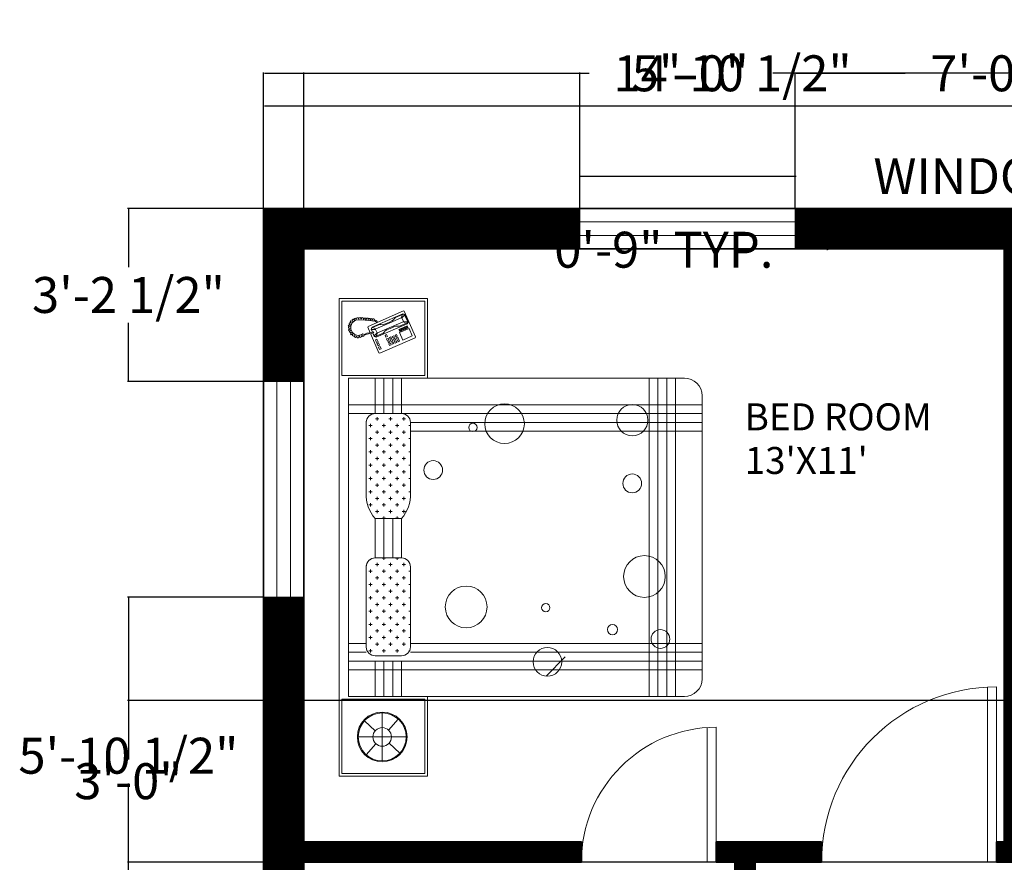
# Model space of a CAD drawing. Units: inches. Extents: x 108 to 771, y 58 to 590.
# Tile 5 of 8: x 108 to 327, y 402 to 590. Entities that reach past the tile are written whole.
import ezdxf

# ---------------------------------------------------------------- set-up
doc = ezdxf.new("R2010")
doc.units = ezdxf.units.IN
doc.header["$MEASUREMENT"] = 0
for name, color, linetype, lineweight in [('A-ANNO-DIMS', 2, 'Continuous', 13), ('A-AREA-IDEN', 7, 'Continuous', 18), ('A-DOOR', 3, 'Continuous', 18), ('A-GLAZ', 4, 'Continuous', 18), ('A-WALL', 7, 'Continuous', 35), ('A-WALL-PATT', 252, 'Continuous', 9), ('Furniture', 7, 'Continuous', 15)]:
    doc.layers.add(name, color=color, linetype=linetype, lineweight=lineweight)
doc.styles.get("Standard").update_dxf_attribs({"font": 'italic8.shx'})
doc.dimstyles.get("Standard").update_dxf_attribs({"dimtxt": 8, "dimasz": 0.18, "dimexe": 0.18, "dimexo": 0.0625, "dimgap": 0.09, "dimtad": 0, "dimtih": 1, "dimtoh": 1, "dimzin": 0, "dimdsep": 46, "dimlunit": 3, "dimtxsty": 'Standard', "dimcen": 0.09, "dimclrt": 6, "dimadec": 0, "dimazin": 0, "dimtfac": 1, "dimtofl": 0, "dimtmove": 0, "dimatfit": 3, "dimfxl": 1, "dimtolj": 1, "dimtzin": 0, "dimarcsym": 0})

# ---------------------------------------------------------------- blocks, each defined once
blk = doc.blocks.new('*D5')
at = {"layer": 'A-ANNO-DIMS', "color": 0, "lineweight": -2, "transparency": 16777216}
for p, q in [((162.35, 548.12), (162.35, 571.05)), ((162.53, 570.87), (386.42, 570.87)), ((677.17, 570.87), (453.27, 570.87)), ((677.35, 548.12), (677.35, 571.05))]:
    blk.add_line(p, q, dxfattribs=at)
at = {"layer": 'A-ANNO-DIMS', "color": 0, "transparency": 16777216}
for points in [[(162.53, 570.9), (162.53, 570.84), (162.35, 570.87)], [(677.17, 570.9), (677.17, 570.84), (677.35, 570.87)]]:
    blk.add_solid(points, dxfattribs=at)
at = {"layer": 'Defpoints', "color": 0, "transparency": 16777216}
for p in [(677.35, 570.87), (162.35, 548.05), (677.35, 548.05)]:
    blk.add_point(p, dxfattribs=at)
at = {"layer": 'A-ANNO-DIMS', "color": 0, "transparency": 16777216, "insert": (419.85, 570.87), "char_height": 8, "attachment_point": 5}
blk.add_mtext('\\A1;42\'-11.00"', dxfattribs=at)
blk = doc.blocks.new('DOOR-SINGLE-39')
for p, q in [((0, 39), (0, 0)), ((2, 38.95), (2, 0)), ((0, 0), (39, 0))]:
    blk.add_line(p, q)
blk.add_arc((0, 0), 39, 0, 90)
blk = doc.blocks.new('DOOR-SINGLE-30')
for p, q in [((28, 29.93), (28, 0)), ((30, 30), (30, 0)), ((30, 0), (0, 0))]:
    blk.add_line(p, q)
blk.add_arc((30, 0), 30, 90, 180)
blk = doc.blocks.new('WINDOW-48')
for p, q in [((0, 48), (0, 0)), ((9, 48), (0, 48)), ((3, 48), (3, 0)), ((6, 48), (6, 0)), ((9, 0), (9, 48)), ((0, 0), (9, 0))]:
    blk.add_line(p, q)
blk = doc.blocks.new('BED-WITH-NIGHTSTANDS')
h = blk.add_hatch()
h.set_pattern_fill('CROSS', color=256, scale=5.9055, angle=450, style=0)
h.set_pattern_definition([(90, (-724.7189, -618.2251), (1.476375, 1.476375), [0.7381875, -2.2145625]), (360, (-725.088, -617.856), (1.476375, -1.476375), [0.7381875, -2.2145625])])
h.paths.add_polyline_path([(13.93, 48.57), (8.02, 48.57, 0.414214), (6.06, 46.6), (6.06, 28.74, 0.414214), (8.02, 26.77), (13.93, 26.77, 0.414214), (15.9, 28.74), (15.9, 46.6, 0.414214)])
h.paths.add_polyline_path([(6.06, 62.99, 0.19223), (8.02, 57.33), (13.93, 57.33, 0.19223), (15.9, 62.99), (15.9, 78.74, 0.414214), (13.93, 80.71), (8.02, 80.71, 0.414214), (6.06, 78.74)])
for p, q in [((0, 0), (0, 106.3)), ((19.69, 106.3), (0, 106.3)), ((19.09, 105.71), (0.59, 105.71)), ((0.59, 105.71), (0.59, 89.17)), ((19.09, 105.71), (19.09, 89.17)), ((19.69, 106.3), (19.69, 88.58)), ((14.35, 103.55), (6.45, 100.09)), ((14.52, 103.48), (14.35, 103.55)), ((17.02, 97.76), (14.52, 103.48)), ((2.23, 100.67), (2.3, 100.88)), ((2.3, 100.88), (2.69, 100.86)), ((2.44, 101.15), (2.63, 101.34)), ((2.69, 100.86), (2.44, 101.15)), ((2.89, 100.92), (2.62, 100.19)), ((2.63, 101.34), (3.06, 101.2)), ((2.89, 101.55), (3.11, 101.7)), ((3.06, 101.2), (2.89, 101.55)), ((3.69, 101.46), (2.89, 100.92)), ((3.11, 101.7), (3.41, 101.48)), ((3.36, 101.88), (3.67, 101.95)), ((3.41, 101.48), (3.36, 101.88)), ((3.67, 101.95), (3.81, 101.64)), ((4.95, 101.56), (3.69, 101.46)), ((3.81, 101.64), (3.94, 101.98)), ((3.94, 101.98), (4.24, 102.02)), ((4.24, 102.02), (4.39, 101.64)), ((4.37, 102.03), (4.76, 102.08)), ((4.39, 101.64), (4.37, 102.03)), ((4.76, 102.08), (4.88, 101.72)), ((4.88, 101.72), (5.13, 102.07)), ((5.79, 101.48), (4.95, 101.56)), ((5.13, 102.07), (5.37, 102.03)), ((5.37, 102.03), (5.42, 101.66)), ((5.42, 101.66), (5.65, 101.97)), ((5.65, 101.97), (5.95, 101.95)), ((5.86, 101.55), (5.79, 101.48)), ((5.92, 101.48), (5.86, 101.55)), ((6.5, 101.45), (5.92, 101.48)), ((5.95, 101.95), (5.98, 101.59)), ((5.98, 101.59), (6.16, 101.92)), ((6.16, 101.92), (6.47, 101.91)), ((6.47, 101.91), (6.46, 101.54)), ((6.46, 101.54), (6.62, 101.9)), ((7.29, 101.35), (6.5, 101.45)), ((6.62, 101.9), (6.85, 101.89)), ((6.85, 101.89), (6.89, 101.51)), ((6.89, 101.51), (7.15, 101.84)), ((7.15, 101.84), (7.36, 101.82)), ((7.73, 101.29), (7.29, 101.35)), ((14.21, 102.94), (7.34, 99.94)), ((7.36, 101.82), (7.4, 101.48)), ((7.4, 101.48), (7.62, 101.8)), ((7.62, 101.8), (7.77, 101.81)), ((7.79, 101.48), (7.73, 101.29)), ((7.77, 101.81), (7.86, 101.7)), ((7.84, 101.37), (7.79, 101.48)), ((7.94, 101.33), (7.84, 101.37)), ((7.86, 101.7), (7.96, 101.49)), ((8.11, 101.22), (7.94, 101.33)), ((7.96, 101.49), (8.25, 101.43)), ((8.26, 101.14), (8.11, 101.22)), ((11.28, 100.91), (8.18, 99.56)), ((8.25, 101.43), (8.4, 101.32)), ((8.4, 100.95), (8.26, 101.14)), ((8.4, 101.32), (8.57, 101.02)), ((10.11, 100.6), (11.2, 101.08)), ((11.77, 101.33), (11.2, 101.08)), ((11.28, 100.91), (13.85, 102.03)), ((11.68, 99.99), (14.25, 101.12)), ((12.15, 101.56), (11.77, 101.33)), ((12.36, 101.86), (12.15, 101.56)), ((12.6, 102.1), (12.36, 101.86)), ((14.14, 102.78), (12.6, 102.1)), ((14.14, 102.78), (13.85, 102.03)), ((13.85, 102.03), (13.99, 102.03)), ((13.99, 102.03), (14.61, 102.64)), ((13.99, 102.03), (14.34, 101.23)), ((14.4, 102.82), (14.14, 102.78)), ((14.62, 102.78), (14.21, 102.94)), ((14.25, 101.12), (14.34, 101.23)), ((15, 100.83), (14.25, 101.12)), ((14.34, 101.23), (15.21, 101.26)), ((14.61, 102.64), (14.4, 102.82)), ((15.21, 101.26), (14.61, 102.64)), ((15.37, 101.06), (14.62, 102.78)), ((15.2, 100.99), (15, 100.83)), ((15.18, 100.71), (15.37, 101.06)), ((15.21, 101.26), (15.2, 100.99)), ((2.06, 100.15), (2.14, 100.41)), ((2.46, 100.04), (2.06, 100.15)), ((2.09, 99.7), (2.1, 99.92)), ((2.44, 99.53), (2.09, 99.7)), ((2.1, 99.92), (2.46, 100.04)), ((2.13, 99.38), (2.44, 99.53)), ((2.17, 99.14), (2.13, 99.38)), ((2.14, 100.41), (2.51, 100.41)), ((2.59, 99.17), (2.17, 99.14)), ((2.51, 100.41), (2.23, 100.67)), ((2.29, 98.95), (2.59, 99.17)), ((2.4, 98.76), (2.29, 98.95)), ((2.78, 98.76), (2.4, 98.76)), ((2.53, 98.47), (2.78, 98.76)), ((2.62, 100.19), (2.62, 99.39)), ((2.62, 99.39), (2.98, 98.72)), ((2.98, 98.72), (3.58, 98.25)), ((6.45, 100.09), (6.38, 99.93)), ((6.38, 99.93), (6.92, 98.7)), ((6.77, 98.66), (7.17, 98.75)), ((7.34, 99.94), (7.12, 99.5)), ((7.12, 99.5), (7.41, 98.83)), ((7.17, 98.75), (7.65, 98.91)), ((7.72, 98.74), (7.22, 98.53)), ((7.23, 99.41), (7.24, 99.69)), ((8.09, 99.45), (7.23, 99.41)), ((7.47, 98.85), (7.23, 99.41)), ((7.24, 99.69), (7.44, 99.85)), ((7.44, 99.85), (8.99, 100.52)), ((7.44, 99.85), (8.18, 99.56)), ((7.65, 98.91), (7.72, 98.74)), ((8.18, 99.56), (8.09, 99.45)), ((8.09, 99.45), (8.45, 98.65)), ((8.26, 97.68), (15.18, 100.71)), ((11.68, 99.99), (8.58, 98.64)), ((8.99, 100.52), (9.33, 100.53)), ((9.33, 100.53), (9.69, 100.49)), ((9.69, 100.49), (10.11, 100.6)), ((9.84, 98.58), (10.08, 98.82)), ((10.08, 98.82), (10.29, 99.11)), ((10.29, 99.11), (10.66, 99.34)), ((10.66, 99.34), (11.75, 99.82)), ((12.33, 100.07), (11.75, 99.82)), ((12.75, 100.19), (12.33, 100.07)), ((13.11, 100.14), (12.75, 100.19)), ((13.45, 100.15), (13.11, 100.14)), ((13.3, 99.4), (13.47, 99.48)), ((13.5, 98.95), (13.3, 99.4)), ((15, 100.83), (13.45, 100.15)), ((15.58, 99.65), (13.46, 98.72)), ((13.46, 98.72), (14.18, 97.06)), ((13.47, 99.48), (13.67, 99.02)), ((13.67, 99.02), (13.5, 98.95)), ((13.64, 99.55), (13.81, 99.63)), ((13.84, 99.1), (13.64, 99.55)), ((13.81, 99.63), (14.01, 99.17)), ((14.01, 99.17), (13.84, 99.1)), ((13.99, 99.7), (14.16, 99.78)), ((14.19, 99.25), (13.99, 99.7)), ((14.16, 99.78), (14.36, 99.32)), ((14.36, 99.32), (14.19, 99.25)), ((14.33, 99.85), (14.5, 99.93)), ((14.53, 99.4), (14.33, 99.85)), ((14.5, 99.93), (14.7, 99.47)), ((14.7, 99.47), (14.53, 99.4)), ((14.67, 100), (14.84, 100.08)), ((14.87, 99.55), (14.67, 100)), ((14.84, 100.08), (15.04, 99.62)), ((15.04, 99.62), (14.87, 99.55)), ((15.02, 100.16), (15.19, 100.23)), ((15.22, 99.7), (15.02, 100.16)), ((15.19, 100.23), (15.39, 99.77)), ((15.39, 99.77), (15.22, 99.7)), ((16.3, 97.99), (15.58, 99.65)), ((2.71, 98.26), (2.53, 98.47)), ((3.07, 98.46), (2.71, 98.26)), ((2.96, 98.08), (3.07, 98.46)), ((3.2, 97.92), (2.96, 98.08)), ((3.49, 98.1), (3.2, 97.92)), ((3.41, 97.75), (3.49, 98.1)), ((3.69, 97.67), (3.41, 97.75)), ((3.58, 98.25), (4.33, 98.05)), ((3.95, 97.97), (3.69, 97.67)), ((4.03, 97.59), (3.95, 97.97)), ((4.36, 97.56), (4.03, 97.59)), ((4.33, 98.05), (5.08, 98.31)), ((4.48, 97.99), (4.36, 97.56)), ((4.67, 97.64), (4.48, 97.99)), ((5, 97.75), (4.67, 97.64)), ((5.05, 98.16), (5, 97.75)), ((5.26, 97.85), (5.05, 98.16)), ((5.08, 98.31), (5.33, 98.48)), ((5.53, 98), (5.26, 97.85)), ((5.33, 98.48), (5.57, 98.34)), ((5.6, 98.18), (5.53, 98)), ((5.57, 98.34), (5.87, 98.48)), ((5.68, 98.18), (5.6, 98.18)), ((5.98, 98.32), (5.68, 98.18)), ((5.87, 98.48), (6.16, 98.57)), ((6.58, 98.42), (5.98, 98.32)), ((6.16, 98.57), (6.77, 98.66)), ((7.22, 98.53), (6.58, 98.42)), ((7.01, 98.5), (8.89, 94.2)), ((7.49, 98.64), (7.84, 97.84)), ((7.83, 98.04), (7.55, 98.67)), ((8.45, 98.65), (7.83, 98.04)), ((7.83, 98.04), (8.04, 97.86)), ((7.84, 97.84), (8.26, 97.68)), ((8.04, 97.86), (8.29, 97.9)), ((8.09, 97.13), (8.43, 97.28)), ((8.34, 96.55), (8.09, 97.13)), ((8.29, 97.9), (8.58, 98.64)), ((8.29, 97.9), (9.84, 98.58)), ((8.68, 96.7), (8.34, 96.55)), ((8.43, 97.28), (8.68, 96.7)), ((8.58, 98.64), (8.45, 98.65)), ((9.05, 94.14), (16.96, 97.59)), ((10.58, 98.29), (10.24, 98.14)), ((10.24, 98.14), (10.44, 97.68)), ((10.44, 97.68), (10.78, 97.83)), ((10.78, 97.83), (10.58, 98.29)), ((10.93, 97.48), (10.59, 97.33)), ((10.59, 97.33), (10.74, 96.99)), ((10.74, 96.99), (11.08, 97.14)), ((11.18, 96.91), (10.84, 96.76)), ((10.84, 96.76), (10.99, 96.42)), ((11.08, 97.14), (10.93, 97.48)), ((10.99, 96.42), (11.33, 96.57)), ((11.33, 96.57), (11.18, 96.91)), ((11.56, 97.76), (11.22, 97.61)), ((11.22, 97.61), (11.37, 97.27)), ((11.37, 97.27), (11.71, 97.42)), ((11.81, 97.19), (11.47, 97.04)), ((11.47, 97.04), (11.62, 96.69)), ((11.71, 97.42), (11.56, 97.76)), ((11.62, 96.69), (11.96, 96.84)), ((12.06, 96.61), (11.72, 96.46)), ((11.96, 96.84), (11.81, 97.19)), ((12.19, 98.03), (11.85, 97.88)), ((11.85, 97.88), (12, 97.54)), ((12, 97.54), (12.34, 97.69)), ((12.21, 96.27), (12.06, 96.61)), ((12.44, 97.46), (12.1, 97.31)), ((12.1, 97.31), (12.25, 96.97)), ((12.34, 97.69), (12.19, 98.03)), ((12.25, 96.97), (12.59, 97.12)), ((12.69, 96.89), (12.35, 96.74)), ((12.35, 96.74), (12.5, 96.39)), ((12.59, 97.12), (12.44, 97.46)), ((12.82, 98.31), (12.48, 98.16)), ((12.48, 98.16), (12.63, 97.82)), ((12.5, 96.39), (12.84, 96.55)), ((12.63, 97.82), (12.97, 97.97)), ((12.84, 96.55), (12.69, 96.89)), ((13.07, 97.74), (12.73, 97.59)), ((12.73, 97.59), (12.88, 97.24)), ((12.97, 97.97), (12.82, 98.31)), ((12.88, 97.24), (13.22, 97.39)), ((13.32, 97.16), (12.98, 97.01)), ((12.98, 97.01), (13.13, 96.67)), ((13.22, 97.39), (13.07, 97.74)), ((13.13, 96.67), (13.47, 96.82)), ((13.47, 96.82), (13.32, 97.16)), ((14.18, 97.06), (16.3, 97.99)), ((16.96, 97.59), (17.02, 97.76)), ((8.44, 96.33), (8.78, 96.48)), ((8.69, 95.75), (8.44, 96.33)), ((9.03, 95.9), (8.69, 95.75)), ((8.78, 96.48), (9.03, 95.9)), ((8.79, 95.52), (9.13, 95.67)), ((9.04, 94.95), (8.79, 95.52)), ((9.38, 95.1), (9.04, 94.95)), ((9.13, 95.67), (9.38, 95.1)), ((11.43, 96.34), (11.09, 96.19)), ((11.09, 96.19), (11.24, 95.84)), ((11.24, 95.84), (11.58, 95.99)), ((11.58, 95.99), (11.43, 96.34)), ((11.72, 96.46), (11.87, 96.12)), ((11.87, 96.12), (12.21, 96.27)), ((8.89, 94.2), (9.05, 94.14)), ((19.09, 89.17), (0.59, 89.17)), ((0.59, 89.17), (19.09, 89.17)), ((2.12, 17.72), (2.12, 88.58)), ((2.12, 88.58), (76.92, 88.58)), ((80.86, 84.65), (80.86, 21.65)), ((55.34, 82.68), (55.28, 82.62)), ((6.07, 78.98), (6.07, 62.76)), ((6.07, 46.84), (6.07, 28.51)), ((6.07, 44.57), (6.06, 44.56)), ((50.36, 26.51), (46.1, 22.26)), ((76.92, 17.72), (2.12, 17.72)), ((19.69, 0), (19.69, 17.72)), ((19.09, 17.13), (0.59, 17.13)), ((0.59, 0.59), (0.59, 17.13)), ((19.09, 0.59), (19.09, 17.13)), ((9.61, 8.71), (9.61, 14.05)), ((8.07, 10.1), (5.65, 12.3)), ((11, 10.24), (13.2, 12.67)), ((9.61, 8.71), (4.26, 8.71)), ((8.22, 7.18), (6.02, 4.75)), ((9.61, 8.71), (14.95, 8.71)), ((9.61, 8.71), (9.61, 3.36)), ((11.14, 7.32), (13.56, 5.12)), ((19.69, 0), (0, 0)), ((19.09, 0.59), (0.59, 0.59))]:
    blk.add_line(p, q)
for points in [[(8.02, 88.58), (8.02, 80.71)], [(9.99, 80.71), (9.99, 88.58), (8.02, 88.58)], [(13.93, 80.71), (13.93, 88.58), (11.96, 88.58)], [(11.96, 88.58), (11.96, 80.71)], [(2.12, 80.71), (80.86, 80.71), (80.86, 82.68), (2.12, 82.68)], [(15.9, 76.77), (80.86, 76.77), (80.86, 78.74), (15.9, 78.74)], [(8.02, 57.33), (8.02, 48.57)], [(9.99, 48.57), (9.99, 57.33)], [(11.96, 57.33), (11.96, 48.57)], [(13.93, 48.57), (13.93, 57.33)], [(2.12, 29.53), (6.06, 29.53)], [(15.9, 29.53), (80.86, 29.53), (80.86, 27.56), (15.9, 27.56)], [(6.06, 27.56), (2.12, 27.56)], [(2.12, 25.59), (80.86, 25.59), (80.86, 23.62), (2.12, 23.62)], [(8.02, 25.59), (8.02, 17.72), (9.99, 17.72), (9.99, 25.59)], [(11.96, 25.59), (11.96, 17.72), (13.93, 17.72), (13.93, 25.59)]]:
    blk.add_lwpolyline(points)
for points in [[(69.05, 88.58), (69.05, 17.72), (71.02, 17.72), (71.02, 88.58)], [(72.98, 88.58), (72.98, 17.72), (74.95, 17.72), (74.95, 88.58)]]:
    blk.add_lwpolyline(points, close=True)
for points in [[(15.9, 62.99), (15.9, 78.74, 0.414214), (13.93, 80.71), (8.02, 80.71, 0.414214), (6.06, 78.74), (6.06, 62.99, 0.19223), (8.02, 57.33), (13.93, 57.33, 0.19223)], [(15.9, 28.74), (15.9, 46.6, 0.414214), (13.93, 48.57), (8.02, 48.57, 0.414214), (6.06, 46.6), (6.06, 28.74, 0.414214), (8.02, 26.77), (13.93, 26.77, 0.414214)]]:
    blk.add_lwpolyline(points, format="xyb", close=True)
for centre, radius in [((36.86, 78.44), 4.41), ((65.32, 79.25), 3.48), ((29.81, 77.62), 0.925), ((20.97, 68.13), 2.09), ((65.3, 65.16), 2.09), ((68.02, 44.43), 4.65), ((28.31, 37.66), 4.65), ((46.05, 37.48), 0.925), ((60.91, 32.6), 1.14), ((71.58, 30.51), 2.09), ((46.4, 25.43), 3.19), ((9.61, 8.71), 5.54), ((9.61, 8.71), 5.34), ((9.61, 8.71), 2.07)]:
    blk.add_circle(centre, radius)
for centre, start, end in [((76.92, 84.65), 0, 90), ((76.92, 21.65), 270, 0)]:
    blk.add_arc(centre, 3.94, start, end)
blk = doc.blocks.new('*D20')
at = {"layer": 'A-ANNO-DIMS', "color": 0, "lineweight": -2, "transparency": 16777216}
for p, q in [((232.77, 548.12), (232.77, 555.43)), ((232.95, 555.25), (280.59, 555.25)), ((280.77, 548.12), (280.77, 555.43)), ((280.77, 555.25), (280.95, 555.25))]:
    blk.add_line(p, q, dxfattribs=at)
at = {"layer": 'A-ANNO-DIMS', "color": 0, "transparency": 16777216}
for points in [[(232.95, 555.28), (232.95, 555.22), (232.77, 555.25)], [(280.59, 555.28), (280.59, 555.22), (280.77, 555.25)]]:
    blk.add_solid(points, dxfattribs=at)
at = {"layer": 'Defpoints', "color": 0, "transparency": 16777216}
for p in [(280.77, 555.25), (232.77, 548.05), (280.77, 548.05)]:
    blk.add_point(p, dxfattribs=at)
at = {"layer": 'A-ANNO-DIMS', "color": 6, "transparency": 16777216, "insert": (346.76, 555.25), "char_height": 8, "attachment_point": 5}
blk.add_mtext('\\A1;WINDOW 4\'-0" TYP.', dxfattribs=at)
blk = doc.blocks.new('*D21')
at = {"layer": 'A-ANNO-DIMS', "color": 0, "lineweight": -2, "transparency": 16777216}
for p, q in [((280.83, 548.05), (288.15, 548.05)), ((287.97, 547.87), (287.97, 539.23)), ((280.83, 539.05), (288.15, 539.05)), ((287.97, 538.87), (287.79, 538.87)), ((287.97, 539.05), (287.97, 538.87))]:
    blk.add_line(p, q, dxfattribs=at)
at = {"layer": 'A-ANNO-DIMS', "color": 0, "transparency": 16777216}
for points in [[(287.94, 547.87), (288, 547.87), (287.97, 548.05)], [(287.94, 539.23), (288, 539.23), (287.97, 539.05)]]:
    blk.add_solid(points, dxfattribs=at)
at = {"layer": 'Defpoints', "color": 0, "transparency": 16777216}
for p in [(280.77, 548.05), (280.77, 539.05), (287.97, 539.05)]:
    blk.add_point(p, dxfattribs=at)
at = {"layer": 'A-ANNO-DIMS', "color": 6, "transparency": 16777216, "insert": (251.51, 538.87), "char_height": 8, "attachment_point": 5}
blk.add_mtext('\\A1;0\'-9" TYP.', dxfattribs=at)
blk = doc.blocks.new('*D53')
at = {"layer": 'A-ANNO-DIMS', "color": 0, "lineweight": -2, "transparency": 16777216}
for p, q in [((162.35, 548.12), (162.35, 578.33)), ((162.53, 578.15), (232.59, 578.15)), ((232.77, 548.12), (232.77, 578.33)), ((232.77, 578.15), (232.95, 578.15))]:
    blk.add_line(p, q, dxfattribs=at)
at = {"layer": 'A-ANNO-DIMS', "color": 0, "transparency": 16777216}
for points in [[(162.53, 578.18), (162.53, 578.12), (162.35, 578.15)], [(232.59, 578.18), (232.59, 578.12), (232.77, 578.15)]]:
    blk.add_solid(points, dxfattribs=at)
at = {"layer": 'Defpoints', "color": 0, "transparency": 16777216}
for p in [(232.77, 578.15), (162.35, 548.05), (232.77, 548.05)]:
    blk.add_point(p, dxfattribs=at)
at = {"layer": 'A-ANNO-DIMS', "color": 6, "transparency": 16777216, "insert": (268.85, 578.15), "char_height": 8, "attachment_point": 5}
blk.add_mtext('\\A1;5\'-10 1/2"', dxfattribs=at)
blk = doc.blocks.new('*D54')
at = {"layer": 'A-ANNO-DIMS', "color": 0, "lineweight": -2, "transparency": 16777216}
for p, q in [((280.77, 548.12), (280.77, 578.33)), ((280.95, 578.15), (305.28, 578.15)), ((364.84, 578.15), (340.51, 578.15)), ((365.02, 548.12), (365.02, 578.33))]:
    blk.add_line(p, q, dxfattribs=at)
at = {"layer": 'A-ANNO-DIMS', "color": 0, "transparency": 16777216}
for points in [[(280.95, 578.18), (280.95, 578.12), (280.77, 578.15)], [(364.84, 578.18), (364.84, 578.12), (365.02, 578.15)]]:
    blk.add_solid(points, dxfattribs=at)
at = {"layer": 'Defpoints', "color": 0, "transparency": 16777216}
for p in [(365.02, 578.15), (280.77, 548.05), (365.02, 548.05)]:
    blk.add_point(p, dxfattribs=at)
at = {"layer": 'A-ANNO-DIMS', "color": 6, "transparency": 16777216, "insert": (322.9, 578.15), "char_height": 8, "attachment_point": 5}
blk.add_mtext('\\A1;7\'-0"', dxfattribs=at)
blk = doc.blocks.new('*D57')
at = {"layer": 'A-ANNO-DIMS', "color": 0, "lineweight": -2, "transparency": 16777216}
for p, q in [((162.28, 548.05), (132.07, 548.05)), ((132.25, 547.87), (132.25, 534.99)), ((132.25, 509.73), (132.25, 522.62)), ((171.28, 509.55), (132.07, 509.55))]:
    blk.add_line(p, q, dxfattribs=at)
at = {"layer": 'A-ANNO-DIMS', "color": 0, "transparency": 16777216}
for points in [[(132.22, 547.87), (132.28, 547.87), (132.25, 548.05)], [(132.22, 509.73), (132.28, 509.73), (132.25, 509.55)]]:
    blk.add_solid(points, dxfattribs=at)
at = {"layer": 'Defpoints', "color": 0, "transparency": 16777216}
for p in [(132.25, 548.05), (162.35, 548.05), (171.35, 509.55)]:
    blk.add_point(p, dxfattribs=at)
at = {"layer": 'A-ANNO-DIMS', "color": 6, "transparency": 16777216, "insert": (132.25, 528.8), "char_height": 8, "attachment_point": 5}
blk.add_mtext('\\A1;3\'-2 1/2"', dxfattribs=at)
blk = doc.blocks.new('*D60')
at = {"layer": 'A-ANNO-DIMS', "color": 0, "lineweight": -2, "transparency": 16777216}
for p, q in [((171.35, 145.12), (171.35, 578.33)), ((171.53, 578.15), (234.87, 578.15)), ((339.17, 578.15), (275.82, 578.15)), ((339.35, 145.12), (339.35, 578.33))]:
    blk.add_line(p, q, dxfattribs=at)
at = {"layer": 'A-ANNO-DIMS', "color": 0, "transparency": 16777216}
for points in [[(171.53, 578.18), (171.53, 578.12), (171.35, 578.15)], [(339.17, 578.18), (339.17, 578.12), (339.35, 578.15)]]:
    blk.add_solid(points, dxfattribs=at)
at = {"layer": 'Defpoints', "color": 0, "transparency": 16777216}
for p in [(339.35, 578.15), (171.35, 145.05), (339.35, 145.05)]:
    blk.add_point(p, dxfattribs=at)
at = {"layer": 'A-ANNO-DIMS', "color": 6, "transparency": 16777216, "insert": (255.35, 578.15), "char_height": 8, "attachment_point": 5}
blk.add_mtext('\\A1;14\'-0"', dxfattribs=at)
blk = doc.blocks.new('*D62')
at = {"layer": 'A-ANNO-DIMS', "color": 0, "lineweight": -2, "transparency": 16777216}
for p, q in [((507.78, 438.55), (132.07, 438.55)), ((132.25, 438.37), (132.25, 425.4)), ((132.25, 402.73), (132.25, 415.7)), ((515.6, 402.55), (132.07, 402.55))]:
    blk.add_line(p, q, dxfattribs=at)
at = {"layer": 'A-ANNO-DIMS', "color": 0, "transparency": 16777216}
for points in [[(132.22, 438.37), (132.28, 438.37), (132.25, 438.55)], [(132.22, 402.73), (132.28, 402.73), (132.25, 402.55)]]:
    blk.add_solid(points, dxfattribs=at)
at = {"layer": 'Defpoints', "color": 0, "transparency": 16777216}
for p in [(507.85, 438.55), (132.25, 402.55), (515.66, 402.55)]:
    blk.add_point(p, dxfattribs=at)
at = {"layer": 'A-ANNO-DIMS', "color": 6, "transparency": 16777216, "insert": (132.25, 420.55), "char_height": 8, "attachment_point": 5}
blk.add_mtext('\\A1;3\'-0"', dxfattribs=at)
blk = doc.blocks.new('*D65')
at = {"layer": 'A-ANNO-DIMS', "color": 0, "lineweight": -2, "transparency": 16777216}
for p, q in [((162.28, 461.55), (132.07, 461.55)), ((132.25, 461.37), (132.25, 432.41)), ((132.25, 391.08), (132.25, 420.04)), ((162.28, 390.9), (132.07, 390.9))]:
    blk.add_line(p, q, dxfattribs=at)
at = {"layer": 'A-ANNO-DIMS', "color": 0, "transparency": 16777216}
for points in [[(132.22, 461.37), (132.28, 461.37), (132.25, 461.55)], [(132.22, 391.08), (132.28, 391.08), (132.25, 390.9)]]:
    blk.add_solid(points, dxfattribs=at)
at = {"layer": 'Defpoints', "color": 0, "transparency": 16777216}
for p in [(132.25, 461.55), (162.35, 461.55), (162.35, 390.9)]:
    blk.add_point(p, dxfattribs=at)
at = {"layer": 'A-ANNO-DIMS', "color": 6, "transparency": 16777216, "insert": (132.25, 426.22), "char_height": 8, "attachment_point": 5}
blk.add_mtext('\\A1;5\'-10 1/2"', dxfattribs=at)

msp = doc.modelspace()

# ---------------------------------------------------------------- hatches: boundary and pattern name
at = {"layer": 'A-WALL-PATT'}
h = msp.add_hatch(dxfattribs=at)
h.set_pattern_fill('ANSI31', color=256)
h.paths.add_polyline_path([(171.345, 461.548), (162.345, 461.548), (162.345, 390.901), (171.345, 390.901), (171.345, 393.51), (171.345, 402.553), (233.142, 402.553), (233.142, 407.053), (171.345, 407.053)])
h.paths.add_polyline_path([(331.845, 438.553), (336.68, 438.554), (336.68, 443.053), (331.845, 443.053), (331.845, 539.053), (365.02, 539.053), (365.02, 548.053), (280.772, 548.053), (280.772, 539.053), (327.345, 539.053), (327.345, 407.053), (325.63, 407.053), (325.63, 402.553), (331.845, 402.553)])
h.paths.add_polyline_path([(286.63, 407.053), (263.142, 407.053), (263.142, 402.553), (267.345, 402.553), (267.345, 352.303), (171.345, 352.303), (171.345, 360.901), (162.345, 360.901), (162.345, 336.026), (171.345, 336.026), (171.345, 347.803), (267.345, 347.803), (267.345, 293.053), (263.142, 293.053), (263.142, 288.553), (293.037, 288.553), (293.037, 293.053), (271.845, 293.053), (271.845, 402.553), (286.63, 402.553)])
h.paths.add_polyline_path([(466.018, 443.053), (424.345, 443.053), (424.345, 539.053), (453.584, 539.053), (453.584, 548.053), (395.02, 548.053), (395.02, 539.053), (419.845, 539.053), (420.71, 443.053), (372.68, 443.053), (372.68, 438.557), (420.751, 438.561), (421.075, 402.553), (422.061, 293.053), (419.994, 293.053), (419.994, 288.553), (426.124, 288.553), (426.124, 293.053), (424.345, 293.053), (424.345, 402.553), (424.345, 438.553), (466.018, 438.553)])
h.paths.add_polyline_path([(512.345, 539.053), (583.918, 539.053), (583.918, 548.053), (483.584, 548.053), (483.584, 539.053), (507.845, 539.053), (507.845, 443.053), (502.018, 443.053), (502.018, 438.553), (507.845, 438.553), (507.845, 402.553), (515.658, 402.553), (515.658, 407.053), (512.345, 407.053)])
h.paths.add_polyline_path([(232.772, 548.053), (162.345, 548.053), (162.345, 509.548), (171.345, 509.548), (171.345, 539.053), (232.772, 539.053)])
h.paths.add_polyline_path([(233.142, 293.053), (171.345, 293.053), (171.345, 306.026), (162.345, 306.026), (162.345, 230.8), (171.345, 230.8), (171.345, 288.553), (233.142, 288.553)])
h.paths.add_polyline_path([(359.994, 293.053), (332.037, 293.053), (332.037, 288.553), (339.345, 288.553), (339.345, 145.053), (334.469, 145.053), (334.469, 136.053), (339.345, 136.053), (339.345, 104.553), (166.845, 104.553), (166.845, 136.053), (211.837, 136.053), (211.837, 145.053), (171.345, 145.053), (171.345, 182.8), (162.345, 182.8), (162.345, 100.053), (343.845, 100.053), (343.845, 136.053), (400.886, 136.053), (400.886, 145.053), (348.345, 145.053), (348.345, 288.553), (359.994, 288.553)])
h.paths.add_polyline_path([(500.345, 288.553), (503.755, 288.553), (503.755, 293.053), (486.124, 293.053), (486.124, 288.553), (491.345, 288.553), (491.345, 145.053), (448.886, 145.053), (448.886, 136.053), (495.845, 136.053), (495.845, 100.053), (677.345, 100.053), (677.345, 186.265), (668.345, 186.265), (668.345, 145.053), (627.637, 145.053), (627.637, 136.053), (672.845, 136.053), (672.845, 104.278), (500.345, 104.539), (500.345, 136.053), (504.239, 136.053), (504.239, 145.053), (500.345, 145.053)])
h.paths.add_polyline_path([(580.913, 293.053), (572.345, 293.053), (572.345, 347.803), (668.345, 347.803), (668.345, 330.831), (677.345, 330.831), (677.345, 366.853), (668.345, 366.853), (668.345, 352.303), (572.345, 352.303), (572.345, 402.553), (580.418, 402.553), (580.418, 407.053), (554.658, 407.053), (554.658, 402.553), (567.845, 402.553), (567.845, 293.053), (542.755, 293.053), (542.755, 288.553), (580.913, 288.553)])
h.paths.add_polyline_path([(677.345, 300.831), (668.345, 300.831), (668.345, 293.053), (610.913, 293.053), (610.913, 288.553), (668.345, 288.553), (668.345, 234.265), (677.345, 234.265)])
h.paths.add_polyline_path([(304.469, 145.053), (259.837, 145.053), (259.837, 136.053), (304.469, 136.053)], flags=17)
h.paths.add_polyline_path([(579.637, 145.053), (534.239, 145.053), (534.239, 136.053), (579.637, 136.053)], flags=17)
h.paths.add_polyline_path([(677.345, 450.416), (668.345, 450.416), (668.345, 407.053), (610.418, 407.053), (610.418, 402.553), (668.345, 402.553), (668.345, 396.853), (677.345, 396.853)])
h.paths.add_polyline_path([(677.345, 548.053), (631.918, 548.053), (631.918, 539.053), (668.345, 539.053), (668.345, 498.416), (677.345, 498.416)])
h = msp.add_hatch(dxfattribs=at)
h.set_pattern_fill('ANSI31', color=256)
h.paths.add_polyline_path([(365.02, 548.053), (280.772, 548.053), (280.772, 539.053), (327.345, 539.053), (327.345, 407.053), (325.63, 407.053), (325.63, 402.553), (331.845, 402.553), (331.845, 438.553), (336.68, 438.554), (336.68, 443.053), (331.845, 443.053), (331.845, 539.053), (365.02, 539.053)])
h.paths.add_polyline_path([(453.584, 548.053), (395.02, 548.053), (395.02, 539.053), (419.845, 539.053), (420.71, 443.053), (372.68, 443.053), (372.68, 438.557), (420.751, 438.561), (421.075, 402.553), (422.061, 293.053), (419.994, 293.053), (419.994, 288.553), (426.124, 288.553), (426.124, 293.053), (424.345, 293.053), (424.345, 402.553), (424.345, 438.553), (466.018, 438.553), (466.018, 443.053), (424.345, 443.053), (424.345, 539.053), (453.584, 539.053)])
h.paths.add_polyline_path([(232.772, 548.053), (162.345, 548.053), (162.345, 509.548), (171.345, 509.548), (171.345, 539.053), (232.772, 539.053)])
h.paths.add_polyline_path([(171.345, 461.548), (162.345, 461.548), (162.345, 390.901), (171.345, 390.901), (171.345, 393.51), (171.345, 402.553), (233.142, 402.553), (233.142, 407.053), (171.345, 407.053)])
h.paths.add_polyline_path([(286.63, 407.053), (263.142, 407.053), (263.142, 402.553), (267.345, 402.553), (267.345, 352.303), (171.345, 352.303), (171.345, 360.901), (162.345, 360.901), (162.345, 336.026), (171.345, 336.026), (171.345, 347.803), (267.345, 347.803), (267.345, 293.053), (263.142, 293.053), (263.142, 288.553), (293.037, 288.553), (293.037, 293.053), (271.845, 293.053), (271.845, 402.553), (286.63, 402.553)])
h.paths.add_polyline_path([(171.345, 306.026), (162.345, 306.026), (162.345, 230.8), (171.345, 230.8), (171.345, 288.553), (233.142, 288.553), (233.142, 293.053), (171.345, 293.053)])
h.paths.add_polyline_path([(348.345, 288.553), (359.994, 288.553), (359.994, 293.053), (332.037, 293.053), (332.037, 288.553), (339.345, 288.553), (339.345, 145.053), (334.469, 145.053), (334.469, 136.053), (339.345, 136.053), (339.345, 104.553), (166.845, 104.553), (166.845, 136.053), (211.837, 136.053), (211.837, 145.053), (171.345, 145.053), (171.345, 182.8), (162.345, 182.8), (162.345, 100.053), (343.845, 100.053), (343.845, 136.053), (400.886, 136.053), (400.886, 145.053), (348.345, 145.053)])
h.paths.add_polyline_path([(503.755, 293.053), (486.124, 293.053), (486.124, 288.553), (491.345, 288.553), (491.345, 145.053), (448.886, 145.053), (448.886, 136.053), (495.845, 136.053), (495.845, 100.053), (677.345, 100.053), (677.345, 186.265), (668.345, 186.265), (668.345, 145.053), (627.637, 145.053), (627.637, 136.053), (672.845, 136.053), (672.845, 104.278), (500.345, 104.539), (500.345, 136.053), (504.239, 136.053), (504.239, 145.053), (500.345, 145.053), (500.345, 288.553), (503.755, 288.553)])
h.paths.add_polyline_path([(580.913, 293.053), (572.345, 293.053), (572.345, 347.803), (668.345, 347.803), (668.345, 330.831), (677.345, 330.831), (677.345, 366.853), (668.345, 366.853), (668.345, 352.303), (572.345, 352.303), (572.345, 402.553), (580.418, 402.553), (580.418, 407.053), (554.658, 407.053), (554.658, 402.553), (567.845, 402.553), (567.845, 293.053), (542.755, 293.053), (542.755, 288.553), (580.913, 288.553)])
h.paths.add_polyline_path([(677.345, 300.831), (668.345, 300.831), (668.345, 293.053), (610.913, 293.053), (610.913, 288.553), (668.345, 288.553), (668.345, 234.265), (677.345, 234.265)])
h.paths.add_polyline_path([(579.637, 145.053), (534.239, 145.053), (534.239, 136.053), (579.637, 136.053)], flags=17)
h.paths.add_polyline_path([(304.469, 145.053), (259.837, 145.053), (259.837, 136.053), (304.469, 136.053)], flags=17)
h.paths.add_polyline_path([(583.918, 548.053), (483.584, 548.053), (483.584, 539.053), (507.845, 539.053), (507.845, 443.053), (502.018, 443.053), (502.018, 438.553), (507.845, 438.553), (507.845, 402.553), (515.658, 402.553), (515.658, 407.053), (512.345, 407.053), (512.345, 539.053), (583.918, 539.053)])
h.paths.add_polyline_path([(677.345, 548.053), (631.918, 548.053), (631.918, 539.053), (668.345, 539.053), (668.345, 498.416), (677.345, 498.416)])
h.paths.add_polyline_path([(677.345, 450.416), (668.345, 450.416), (668.345, 407.053), (610.418, 407.053), (610.418, 402.553), (668.345, 402.553), (668.345, 396.853), (677.345, 396.853)])

# ---------------------------------------------------------------- linework, layer by layer
at = {"layer": 'A-WALL'}
for p, q in [((162.345, 548.053), (677.345, 548.053)), ((162.345, 100.053), (162.345, 548.053)), ((171.345, 539.053), (327.345, 539.053)), ((171.345, 407.053), (171.345, 539.053)), ((327.345, 407.053), (327.345, 539.053)), ((171.345, 407.053), (233.142, 407.053)), ((233.142, 407.053), (233.142, 402.553)), ((263.142, 407.053), (263.142, 402.553)), ((263.142, 407.053), (286.63, 407.053)), ((286.63, 407.053), (286.63, 402.553)), ((325.63, 407.053), (325.63, 402.553)), ((325.63, 407.053), (327.345, 407.053)), ((171.345, 402.553), (233.142, 402.553)), ((171.345, 352.303), (171.345, 402.553)), ((263.142, 402.553), (267.345, 402.553)), ((267.345, 352.303), (267.345, 402.553)), ((271.845, 293.053), (271.845, 402.553)), ((271.845, 402.553), (286.63, 402.553)), ((325.63, 402.553), (331.845, 402.553))]:
    msp.add_line(p, q, dxfattribs=at)

# ---------------------------------------------------------------- block references
at = {"layer": 'A-DOOR', "extrusion": (0, 0, -1), "zscale": -1}
msp.add_blockref('DOOR-SINGLE-39', (-325.63, 402.553), dxfattribs=at)
at = {"layer": 'A-DOOR'}
msp.add_blockref('DOOR-SINGLE-30', (233.142, 402.553), dxfattribs=at)
at = {"layer": 'A-GLAZ'}
for p, rotation in [((232.772, 548.053), 269.9999999999998), ((171.346, 509.547), 180)]:
    msp.add_blockref('WINDOW-48', p, dxfattribs=dict(at, rotation=rotation))
at = {"layer": 'Furniture'}
msp.add_blockref('BED-WITH-NIGHTSTANDS', (179.174, 421.693), dxfattribs=at)

# ---------------------------------------------------------------- texts
at = {"layer": 'A-AREA-IDEN'}
for s, p in [('BED ROOM', (269.529, 498.666)), ("13'X11'", (269.529, 488.952))]:
    msp.add_text(s, height=6, dxfattribs=at).set_placement(p)

# ---------------------------------------------------------------- dimensions: what is measured, and where the dimension line sits
at = {"layer": 'A-ANNO-DIMS'}
for base, p1, p2, override, picture, middle in [((232.772, 578.153), (162.345, 548.053), (232.772, 548.053), {"dimdec": 1, "dimlfac": 1, "dimrnd": 0, "dimzin": 1, "dimdsep": 46, "dimlunit": 4, "dimfrac": 2}, '*D53', (268.851, 578.153)), ((339.345, 578.153), (171.345, 145.053), (339.345, 145.053), {"dimdec": 1, "dimlfac": 1, "dimrnd": 0, "dimzin": 1, "dimdsep": 46, "dimlunit": 4, "dimfrac": 2}, '*D60', (255.345, 578.153)), ((365.02, 578.153), (280.772, 548.053), (365.02, 548.053), {"dimdec": 1, "dimlfac": 1, "dimrnd": 0, "dimzin": 1, "dimdsep": 46, "dimlunit": 4, "dimfrac": 2}, '*D54', (322.896, 578.153)), ((677.345, 570.871), (162.345, 548.053), (677.345, 548.053), {"dimclrd": 0, "dimclre": 0, "dimclrt": 0}, '*D5', (419.845, 570.871))]:
    dim = msp.add_linear_dim(base=base, p1=p1, p2=p2, dimstyle='Standard', override=override, dxfattribs=at)
    dim.commit()
    dim.dimension.update_dxf_attribs({"geometry": picture, "text_midpoint": middle})
dim = msp.add_linear_dim(base=(280.772, 555.253), p1=(232.772, 548.053), p2=(280.772, 548.053), text='WINDOW <> TYP.', dimstyle='Standard', override={"dimdec": 1, "dimlfac": 1, "dimrnd": 0, "dimzin": 1, "dimdsep": 46, "dimlunit": 4, "dimfrac": 2}, dxfattribs=at)
dim.commit()
dim.dimension.update_dxf_attribs({"geometry": '*D20', "text_midpoint": (346.756, 555.253)})
dim = msp.add_linear_dim(base=(287.972, 539.053), p1=(280.772, 548.053), p2=(280.772, 539.053), angle=270, text='<> TYP.', dimstyle='Standard', override={"dimdec": 1, "dimlfac": 1, "dimrnd": 0, "dimzin": 1, "dimdsep": 46, "dimlunit": 4, "dimfrac": 2}, dxfattribs=at)
dim.commit()
dim.dimension.update_dxf_attribs({"geometry": '*D21', "text_midpoint": (251.511, 538.873)})
for base, p1, p2, picture, middle in [((132.245, 548.053), (171.345, 509.548), (162.345, 548.053), '*D57', (132.245, 528.8)), ((132.245, 461.548), (162.345, 390.901), (162.345, 461.548), '*D65', (132.245, 426.225)), ((132.245, 402.553), (507.845, 438.553), (515.658, 402.553), '*D62', (132.245, 420.553))]:
    dim = msp.add_linear_dim(base=base, p1=p1, p2=p2, angle=90, dimstyle='Standard', override={"dimdec": 1, "dimlfac": 1, "dimrnd": 0, "dimzin": 1, "dimdsep": 46, "dimlunit": 4, "dimfrac": 2}, dxfattribs=at)
    dim.commit()
    dim.dimension.update_dxf_attribs({"geometry": picture, "text_midpoint": middle})

doc.saveas('drawing.dxf')
